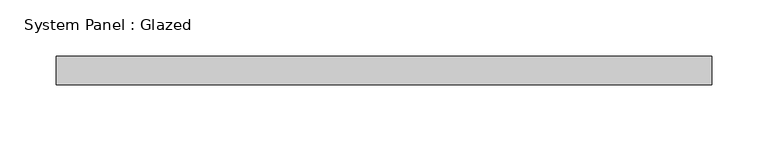
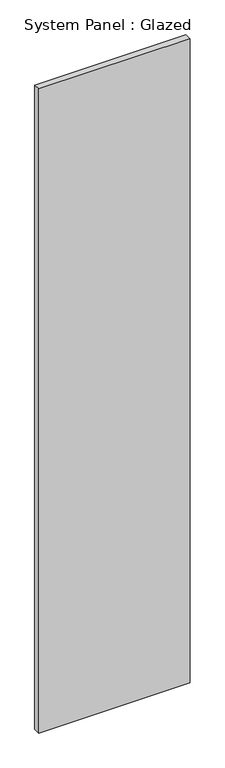
"""IFC4 building model written with IfcOpenShell, lengths in millimetres: plate geometry, System Panel : Glazed."""

from ifc_helpers import new_model, si_unit, origin, origin_with_axes, place, context, project, spatial, polyline, outline, extrude, source, transform, mapped, element, save


def system_panel_glazed_aba10d55(model_context):
    return source(origin(), model_context, "Body", "SweptSolid", [
        extrude(outline(polyline([(291.0416667, 19.05), (-291.0416667, 19.05), (-291.0416667, 44.45), (291.0416667, 44.45), (291.0416667, 19.05)])), origin_with_axes(), (0.0, 0.0, 1.0), 2616.2),
    ])


if __name__ == "__main__":
    model = new_model("IFC4")
    model_context = context("Model", 3, world=origin())
    ifc_project = project(units=[si_unit("LENGTHUNIT", "METRE", prefix="MILLI")], contexts=[model_context])
    site = spatial("IfcSite", under=ifc_project)
    building = spatial("IfcBuilding", under=site)
    placement = place(None, origin())
    system_panel_glazed_shape = system_panel_glazed_aba10d55(model_context)
    element("IfcPlate", 1, ObjectType="System Panel : Glazed", at=placement, inside=building, context=model_context, shape_type="MappedRepresentation", body=[
        mapped(system_panel_glazed_shape, transform((0.0, 0.0, 0.0), x_axis=(1.0, 0.0, 0.0), y_axis=(0.0, 1.0, 0.0), z_axis=(0.0, 0.0, 1.0))),
    ])
    save(model, "model.ifc")

# Revit data of these elements
# Type "System Panel : Glazed"
#   Construction Type Id = "GSP4R"
#   Analytic Construction = "1/8 in Pilkington single glazing"
#   Visual Light Transmittance = 0.9
#   Solar Heat Gain Coefficient = 0.86
#   Heat Transfer Coefficient (U) = 1.18115 BTU/(h·ft²·°F)
#   Define Thermal Properties by = 1
# Element 1 (IfcPlate, "System Panel : Glazed")
#   Materials on its faces: "Glass"
# Materials
#   "Glass": class "Glass", colour RGB 0 128 192, transparency 0.75, Description = "Soda Lime Glass", Cost = 0
